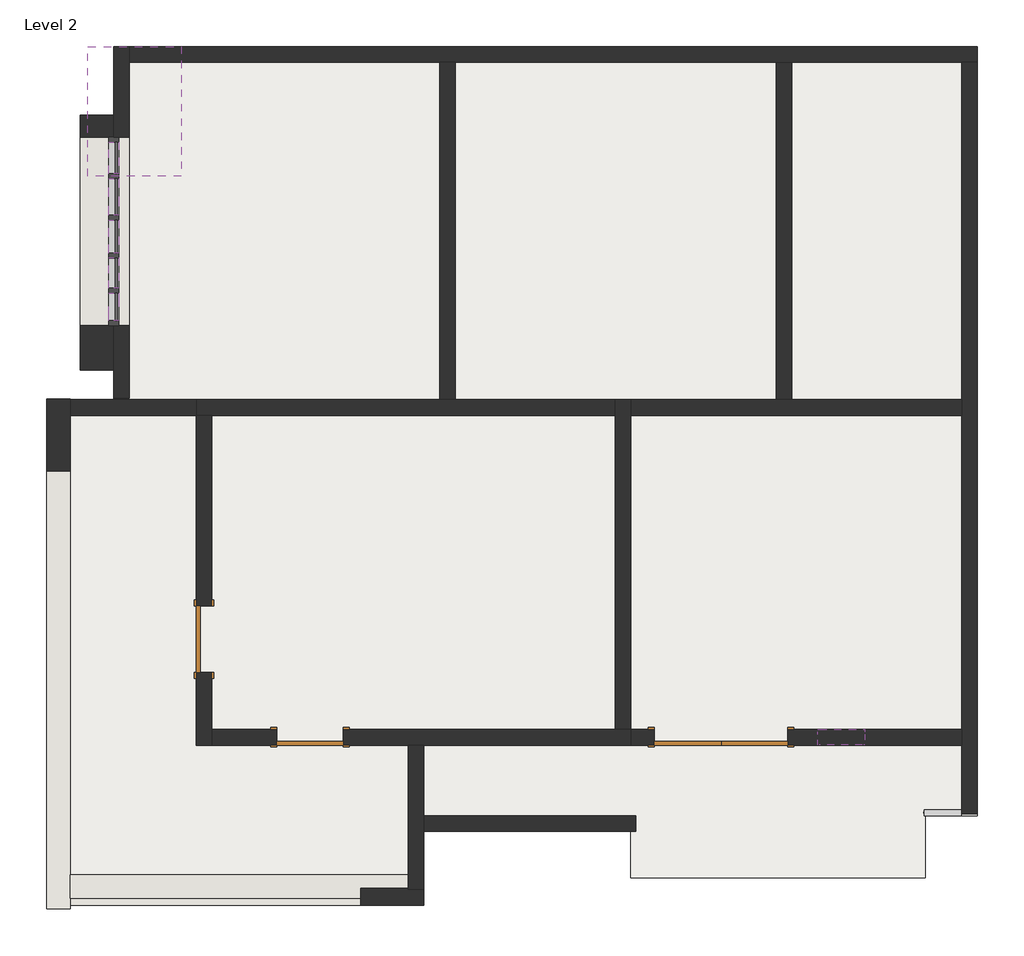
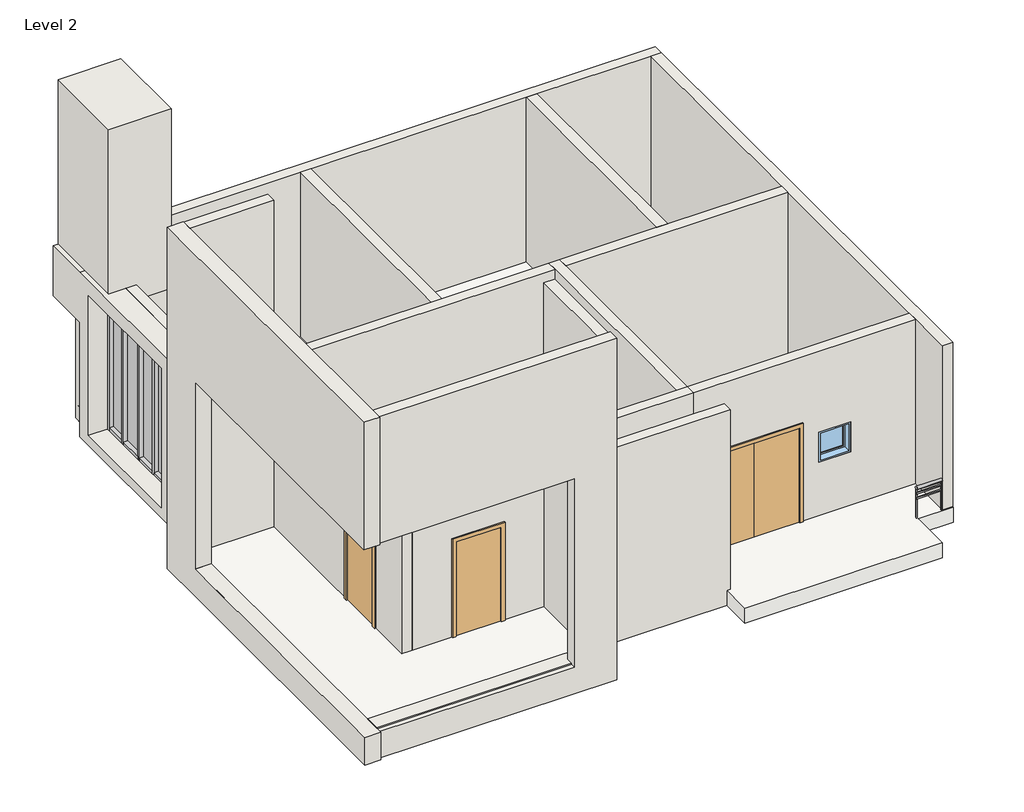
# One storey, incomplete: 19 walls, 16 members, 5 plates, 3 doors, 1 railing, 1 roof, 1 window.
"""IFC4 building model written with IfcOpenShell, lengths in millimetres."""

from ifc_helpers import new_model, si_unit, point, frame, origin, place, context, project, spatial, polyline, ellipse_curve, trimmed, outline, extrude, faceted_brep, transform, mapped, element, save
from ifc_brep_helpers import plane_surface, extruded_surface, advanced_brep
from components import door_aae36eb6, door_ef9e9df2, member_dc106669, member_39486dda, member_2b79973d, member_de12f0f3, member_76ec7c80, member_ae973821, member_2680e53c, system_panel_glazed_213fa7e9, system_panel_glazed_fd82e51e, system_panel_glazed_76cbe525, system_panel_glazed_7e745cad, system_panel_glazed_6096bcca, walls_1_walls_1_c089fa37, walls_2_walls_2_432dc62d, walls_3_walls_3_a2c954b4, walls_4_walls_4_aecb3609, walls_5_walls_5_067f5539, window_6846e476

model = new_model("IFC4")

# Units and contexts
model_context = context("Model", 3, world=origin())
ifc_project = project(units=[si_unit("LENGTHUNIT", "METRE", prefix="MILLI")], contexts=[model_context])

# Site, building, storey
site = spatial("IfcSite", under=ifc_project)
building = spatial("IfcBuilding", under=site)
storey = spatial("IfcBuildingStorey", under=building, Name="Level 2", Elevation=3657.6)

# Doors
placement = place(None, origin())
door_shape = door_aae36eb6(model_context)
element("IfcDoor", 1, ObjectType="Door-Double-Flush_Panel : 68\" x 80\"", at=placement, inside=storey, context=model_context, shape_type="MappedRepresentation", body=[
    mapped(door_shape, transform((-3927.8833771, 2417.2609482, 3860.8), x_axis=(-1.0, 0.0, 0.0), y_axis=(0.0, -1.0, 0.0), z_axis=(0.0, 0.0, 1.0))),
])
door_2_shape = door_ef9e9df2(model_context)
element("IfcDoor", 2, ObjectType="Single-Flush : 34\" x 80\"", at=placement, inside=storey, context=model_context, shape_type="MappedRepresentation", body=[
    mapped(door_2_shape, transform((-10617.8932708, 3687.2609482, 3860.8), x_axis=(0.0, 1.0, 0.0), y_axis=(-1.0, 0.0, 0.0), z_axis=(0.0, 0.0, 1.0))),
])
element("IfcDoor", 3, ObjectType="Single-Flush : 34\" x 80\"", at=placement, inside=storey, context=model_context, shape_type="MappedRepresentation", body=[
    mapped(door_2_shape, transform((-9246.2932708, 2417.2609482, 3860.8), x_axis=(-1.0, 0.0, 0.0), y_axis=(0.0, -1.0, 0.0), z_axis=(0.0, 0.0, 1.0))),
])

# Members
member_shape = member_dc106669(model_context)
element("IfcMember", 4, ObjectType="Rectangular Mullion : 2.5\" x 5\" rectangular", at=placement, inside=storey, context=model_context, shape_type="MappedRepresentation", body=[
    mapped(member_shape, transform((-11786.2932708, 10123.5597172, 4163.611227), x_axis=(0.0, 0.0, -1.0), y_axis=(-1.0, 0.0, 0.0), z_axis=(0.0, 1.0, 0.0))),
])
member_2_shape = member_39486dda(model_context)
element("IfcMember", 5, ObjectType="Rectangular Mullion : 2.5\" x 5\" rectangular", at=placement, inside=storey, context=model_context, shape_type="MappedRepresentation", body=[
    mapped(member_2_shape, transform((-11786.2932708, 9113.9097172, 4163.611227), x_axis=(0.0, 0.0, -1.0), y_axis=(-1.0, 0.0, 0.0), z_axis=(0.0, 1.0, 0.0))),
])
member_3_shape = member_2b79973d(model_context)
element("IfcMember", 6, ObjectType="Rectangular Mullion : 2.5\" x 5\" rectangular", at=placement, inside=storey, context=model_context, shape_type="MappedRepresentation", body=[
    mapped(member_3_shape, transform((-11786.2932708, 9647.3097172, 4163.611227), x_axis=(0.0, 0.0, -1.0), y_axis=(-1.0, 0.0, 0.0), z_axis=(0.0, 1.0, 0.0))),
])
member_4_shape = member_de12f0f3(model_context)
element("IfcMember", 7, ObjectType="Rectangular Mullion : 2.5\" x 5\" rectangular", at=placement, inside=storey, context=model_context, shape_type="MappedRepresentation", body=[
    mapped(member_4_shape, transform((-11786.2932708, 8622.8430505, 4163.611227), x_axis=(0.0, 0.0, -1.0), y_axis=(-1.0, 0.0, 0.0), z_axis=(0.0, 1.0, 0.0))),
])
member_5_shape = member_76ec7c80(model_context)
element("IfcMember", 8, ObjectType="Rectangular Mullion : 2.5\" x 5\" rectangular", at=placement, inside=storey, context=model_context, shape_type="MappedRepresentation", body=[
    mapped(member_5_shape, transform((-11786.2932708, 8169.8763839, 4163.611227), x_axis=(0.0, 0.0, -1.0), y_axis=(-1.0, 0.0, 0.0), z_axis=(0.0, 1.0, 0.0))),
])
member_6_shape = member_ae973821(model_context)
element("IfcMember", 9, ObjectType="Rectangular Mullion : 2.5\" x 5\" rectangular", at=placement, inside=storey, context=model_context, shape_type="MappedRepresentation", body=[
    mapped(member_6_shape, transform((-11786.2932708, 9679.0597172, 4163.611227), x_axis=(0.0, -1.0, 0.0), y_axis=(-1.0, 0.0, 0.0), z_axis=(0.0, 0.0, -1.0))),
])
element("IfcMember", 10, ObjectType="Rectangular Mullion : 2.5\" x 5\" rectangular", at=placement, inside=storey, context=model_context, shape_type="MappedRepresentation", body=[
    mapped(member_6_shape, transform((-11786.2932708, 8654.5930505, 4163.611227), x_axis=(0.0, -1.0, 0.0), y_axis=(-1.0, 0.0, 0.0), z_axis=(0.0, 0.0, -1.0))),
])
element("IfcMember", 11, ObjectType="Rectangular Mullion : 2.5\" x 5\" rectangular", at=placement, inside=storey, context=model_context, shape_type="MappedRepresentation", body=[
    mapped(member_6_shape, transform((-11786.2932708, 9145.6597172, 4163.611227), x_axis=(0.0, -1.0, 0.0), y_axis=(-1.0, 0.0, 0.0), z_axis=(0.0, 0.0, -1.0))),
])
element("IfcMember", 12, ObjectType="Rectangular Mullion : 2.5\" x 5\" rectangular", at=placement, inside=storey, context=model_context, shape_type="MappedRepresentation", body=[
    mapped(member_6_shape, transform((-11786.2932708, 8201.6263839, 4163.611227), x_axis=(0.0, -1.0, 0.0), y_axis=(-1.0, 0.0, 0.0), z_axis=(0.0, 0.0, -1.0))),
])
element("IfcMember", 13, ObjectType="Rectangular Mullion : 2.5\" x 5\" rectangular", at=placement, inside=storey, context=model_context, shape_type="MappedRepresentation", body=[
    mapped(member_4_shape, transform((-11786.2932708, 8233.3763839, 7010.4), x_axis=(0.0, 0.0, 1.0), y_axis=(-1.0, 0.0, 0.0), z_axis=(0.0, -1.0, 0.0))),
])
element("IfcMember", 14, ObjectType="Rectangular Mullion : 2.5\" x 5\" rectangular", at=placement, inside=storey, context=model_context, shape_type="MappedRepresentation", body=[
    mapped(member_2_shape, transform((-11786.2932708, 8686.3430505, 7010.4), x_axis=(0.0, 0.0, 1.0), y_axis=(-1.0, 0.0, 0.0), z_axis=(0.0, -1.0, 0.0))),
])
element("IfcMember", 15, ObjectType="Rectangular Mullion : 2.5\" x 5\" rectangular", at=placement, inside=storey, context=model_context, shape_type="MappedRepresentation", body=[
    mapped(member_3_shape, transform((-11786.2932708, 9177.4097172, 7010.4), x_axis=(0.0, 0.0, 1.0), y_axis=(-1.0, 0.0, 0.0), z_axis=(0.0, -1.0, 0.0))),
])
element("IfcMember", 16, ObjectType="Rectangular Mullion : 2.5\" x 5\" rectangular", at=placement, inside=storey, context=model_context, shape_type="MappedRepresentation", body=[
    mapped(member_shape, transform((-11786.2932708, 9710.8097172, 7010.4), x_axis=(0.0, 0.0, 1.0), y_axis=(-1.0, 0.0, 0.0), z_axis=(0.0, -1.0, 0.0))),
])
element("IfcMember", 17, ObjectType="Rectangular Mullion : 2.5\" x 5\" rectangular", at=placement, inside=storey, context=model_context, shape_type="MappedRepresentation", body=[
    mapped(member_5_shape, transform((-11786.2932708, 7812.1597172, 7010.4), x_axis=(0.0, 0.0, 1.0), y_axis=(-1.0, 0.0, 0.0), z_axis=(0.0, -1.0, 0.0))),
])
member_7_shape = member_2680e53c(model_context)
element("IfcMember", 18, ObjectType="Rectangular Mullion : 2.5\" x 5\" rectangular", at=placement, inside=storey, context=model_context, shape_type="MappedRepresentation", body=[
    mapped(member_7_shape, transform((-11786.2932708, 10187.0597172, 7010.4), x_axis=(0.0, 1.0, 0.0), y_axis=(-1.0, 0.0, 0.0), z_axis=(0.0, 0.0, 1.0))),
])
element("IfcMember", 19, ObjectType="Rectangular Mullion : 2.5\" x 5\" rectangular", at=placement, inside=storey, context=model_context, shape_type="MappedRepresentation", body=[
    mapped(member_7_shape, transform((-11786.2932708, 7748.6597172, 4163.611227), x_axis=(0.0, -1.0, 0.0), y_axis=(-1.0, 0.0, 0.0), z_axis=(0.0, 0.0, -1.0))),
])

# Plates
system_panel_glazed_shape = system_panel_glazed_213fa7e9(model_context)
element("IfcPlate", 20, ObjectType="System Panel : Glazed", at=placement, inside=storey, context=model_context, shape_type="MappedRepresentation", body=[
    mapped(system_panel_glazed_shape, transform((-11786.2932708, 9917.1847172, 4227.111227), x_axis=(0.0, -1.0, 0.0), y_axis=(1.0, 0.0, 0.0), z_axis=(0.0, 0.0, 1.0))),
])
system_panel_glazed_2_shape = system_panel_glazed_fd82e51e(model_context)
element("IfcPlate", 21, ObjectType="System Panel : Glazed", at=placement, inside=storey, context=model_context, shape_type="MappedRepresentation", body=[
    mapped(system_panel_glazed_2_shape, transform((-11786.2932708, 9412.3597172, 4227.111227), x_axis=(0.0, -1.0, 0.0), y_axis=(1.0, 0.0, 0.0), z_axis=(0.0, 0.0, 1.0))),
])
system_panel_glazed_3_shape = system_panel_glazed_76cbe525(model_context)
element("IfcPlate", 22, ObjectType="System Panel : Glazed", at=placement, inside=storey, context=model_context, shape_type="MappedRepresentation", body=[
    mapped(system_panel_glazed_3_shape, transform((-11786.2932708, 8900.1263839, 4227.111227), x_axis=(0.0, -1.0, 0.0), y_axis=(1.0, 0.0, 0.0), z_axis=(0.0, 0.0, 1.0))),
])
system_panel_glazed_4_shape = system_panel_glazed_7e745cad(model_context)
element("IfcPlate", 23, ObjectType="System Panel : Glazed", at=placement, inside=storey, context=model_context, shape_type="MappedRepresentation", body=[
    mapped(system_panel_glazed_4_shape, transform((-11786.2932708, 8428.1097172, 4227.111227), x_axis=(0.0, -1.0, 0.0), y_axis=(1.0, 0.0, 0.0), z_axis=(0.0, 0.0, 1.0))),
])
system_panel_glazed_5_shape = system_panel_glazed_6096bcca(model_context)
element("IfcPlate", 24, ObjectType="System Panel : Glazed", at=placement, inside=storey, context=model_context, shape_type="MappedRepresentation", body=[
    mapped(system_panel_glazed_5_shape, transform((-11786.2932708, 7991.0180505, 4227.111227), x_axis=(0.0, -1.0, 0.0), y_axis=(1.0, 0.0, 0.0), z_axis=(0.0, 0.0, 1.0))),
])

# Railing
element("IfcRailing", 25, ObjectType="Glass Panel - Bottom Fill", at=placement, inside=storey, context=model_context, shape_type="SolidModel", body=[
    advanced_brep(
    [(-818.4208756, 1401.4180656, 4572.0), (-818.4208756, 1477.6180656, 4572.0), (-1301.0208756, 1401.4180656, 4572.0), (-1301.0208756, 1477.6180656, 4572.0)],
    [
        (0, 1, ellipse_curve(frame((-818.4208756, 1439.5180656, 4572.0), z_axis=(1.0, 0.0, 0.0), x_axis=(0.0, 1.0, 0.0)), 38.1, 28.575)),
        (1, 0, ellipse_curve(frame((-818.4208756, 1439.5180656, 4572.0), z_axis=(1.0, 0.0, 0.0), x_axis=(0.0, 1.0, 0.0)), 38.1, 28.575)),
        (2, 3, ellipse_curve(frame((-1301.0208756, 1439.5180656, 4572.0), z_axis=(-1.0, 0.0, 0.0), x_axis=(0.0, 1.0, 0.0)), 38.1, 28.575)),
        (3, 2, ellipse_curve(frame((-1301.0208756, 1439.5180656, 4572.0), z_axis=(-1.0, 0.0, 0.0), x_axis=(0.0, 1.0, 0.0)), 38.1, 28.575)),
        (0, 2),
        (3, 1),
    ],
    [
        plane_surface(frame((-818.4208756, 1439.5180656, 4572.0), z_axis=(1.0, 0.0, 0.0), x_axis=(0.0, -1.0, 0.0))),
        plane_surface(frame((-1301.0208756, 1439.5180656, 4572.0), z_axis=(-1.0, 0.0, 0.0), x_axis=(0.0, -1.0, 0.0))),
        extruded_surface(trimmed(ellipse_curve(frame((-1301.0208756, 1439.5180656, 4572.0), z_axis=(1.0, 0.0, 0.0), x_axis=(0.0, 1.0, 0.0)), 38.1, 28.575), [point((-1301.0208756, 1401.4180656, 4572.0))], [point((-1301.0208756, 1477.6180656, 4572.0))], True, "CARTESIAN"), (482.5999999999999, 0.0, 0.0), 482.5999999999999),
        extruded_surface(trimmed(ellipse_curve(frame((-1301.0208756, 1439.5180656, 4572.0), z_axis=(1.0, 0.0, 0.0), x_axis=(0.0, 1.0, 0.0)), 38.1, 28.575), [point((-1301.0208756, 1477.6180656, 4572.0))], [point((-1301.0208756, 1401.4180656, 4572.0))], True, "CARTESIAN"), (482.5999999999999, 0.0, 0.0), 482.5999999999999),
    ],
    [
        (0, [[1, 2]]),
        (1, [[3, 4]]),
        (2, [[-1, 5, -4, 6]]),
        (3, [[-2, -6, -3, -5]]),
    ],
),
    extrude(outline(polyline([(-818.4208756, 1452.2180656), (-818.4208756, 1426.8180656), (-1301.0208756, 1426.8180656), (-1301.0208756, 1452.2180656), (-818.4208756, 1452.2180656)])), frame((0.0, 0.0, 4457.7), z_axis=(0.0, 0.0, 1.0), x_axis=(1.0, 0.0, 0.0)), (0.0, 0.0, 1.0), 25.4),
    extrude(outline(polyline([(-818.4208756, 1452.2180656), (-818.4208756, 1426.8180656), (-1301.0208756, 1426.8180656), (-1301.0208756, 1452.2180656), (-818.4208756, 1452.2180656)])), frame((0.0, 0.0, 4356.1), z_axis=(0.0, 0.0, 1.0), x_axis=(1.0, 0.0, 0.0)), (0.0, 0.0, 1.0), 25.4),
    extrude(outline(polyline([(-1288.3208756, 1449.0430656), (-1288.3208756, 1429.9930656), (-1307.3708756, 1429.9930656), (-1307.3708756, 1449.0430656), (-1288.3208756, 1449.0430656)])), frame((0.0, 0.0, 3657.6), z_axis=(0.0, 0.0, 1.0), x_axis=(1.0, 0.0, 0.0)), (0.0, 0.0, 1.0), 885.6788223),
    extrude(outline(polyline([(-812.0708756, 1449.0430656), (-812.0708756, 1429.9930656), (-831.1208756, 1429.9930656), (-831.1208756, 1449.0430656), (-812.0708756, 1449.0430656)])), frame((0.0, 0.0, 3657.6), z_axis=(0.0, 0.0, 1.0), x_axis=(1.0, 0.0, 0.0)), (0.0, 0.0, 1.0), 885.6788223),
])

# Roof
element("IfcRoof", 26, ObjectType="Generic - 12\"", at=placement, inside=storey, context=model_context, shape_type="SweptSolid", body=[
    extrude(outline(polyline([(-11786.2932708, 11358.0609482), (-610.2932708, 11358.0609482), (-610.2932708, 1401.2609482), (-1286.2833771, 1401.2609482), (-1286.2833771, 600.2635335), (-5096.2833771, 600.2635335), (-5096.2833771, 1401.2609482), (-7773.0932708, 1401.2609482), (-7773.0932708, 639.2609482), (-12345.0932708, 639.2609482), (-12345.0932708, 6786.0609482), (-11786.2932708, 6786.0609482), (-11786.2932708, 11358.0609482)])), frame((0.0, 0.0, 3657.6), z_axis=(0.0, 0.0, 1.0), x_axis=(1.0, 0.0, 0.0)), (0.0, 0.0, 1.0), 304.8),
])

# Walls
element("IfcWall", 27, ObjectType="Generic - 8\"", at=placement, inside=storey, context=model_context, shape_type="SweptSolid", body=[
    extrude(outline(polyline([(-5032.7833771, 1198.0609482), (-7773.0932708, 1198.0609482), (-7773.0932708, 1401.2609482), (-5032.7833771, 1401.2609482), (-5032.7833771, 1198.0609482)])), frame((0.0, 0.0, 3657.6), z_axis=(0.0, 0.0, 1.0), x_axis=(1.0, 0.0, 0.0)), (0.0, 0.0, 1.0), 3962.4),
])
element("IfcWall", 28, ObjectType="Generic - 8\"", at=placement, inside=storey, context=model_context, shape_type="Brep", body=[
    faceted_brep([(-10719.4932708, 6582.8609482, 3657.6), (-10719.4932708, 2315.6609482, 3657.6), (-10719.4932708, 2315.6609482, 7315.2), (-10719.4932708, 6582.8609482, 7315.2), (-10719.4932708, 3255.4609482, 3860.8), (-10719.4932708, 4119.0609482, 3860.8), (-10719.4932708, 4119.0609482, 5892.8), (-10719.4932708, 3255.4609482, 5892.8), (-10516.2932708, 6582.8609482, 3657.6), (-10516.2932708, 6582.8609482, 7315.2), (-10516.2932708, 2518.8609482, 7315.2), (-10516.2932708, 2315.6609482, 7315.2), (-10516.2932708, 2315.6609482, 3657.6), (-10516.2932708, 2518.8609482, 3657.6), (-10516.2932708, 3255.4609482, 3860.8), (-10516.2932708, 3255.4609482, 5892.8), (-10516.2932708, 4119.0609482, 5892.8), (-10516.2932708, 4119.0609482, 3860.8)], [[[0, 1, 2, 3], [4, 5, 6, 7]], [[8, 9, 10, 11, 12, 13], [14, 15, 16, 17]], [[1, 0, 8, 13, 12]], [[2, 1, 12, 11]], [[0, 3, 9, 8]], [[3, 2, 11, 10, 9]], [[5, 4, 14, 17]], [[6, 5, 17, 16]], [[7, 6, 16, 15]], [[4, 7, 15, 14]]]),
])
element("IfcWall", 29, ObjectType="Generic - 8\"", at=placement, inside=storey, context=model_context, shape_type="Brep", body=[
    faceted_brep([(-10516.2932708, 2315.6609482, 3657.6), (-7976.2932708, 2315.6609482, 3657.6), (-7773.0932708, 2315.6609482, 3657.6), (-5096.2833771, 2315.6609482, 3657.6), (-5096.2833771, 2315.6609482, 7315.2), (-10516.2932708, 2315.6609482, 7315.2), (-8814.4932708, 2315.6609482, 3860.8), (-9678.0932708, 2315.6609482, 3860.8), (-9678.0932708, 2315.6609482, 5892.8), (-8814.4932708, 2315.6609482, 5892.8), (-10516.2932708, 2518.8609482, 3657.6), (-10516.2932708, 2518.8609482, 7315.2), (-5299.4833771, 2518.8609482, 7315.2), (-5096.2833771, 2518.8609482, 7315.2), (-5096.2833771, 2518.8609482, 3657.6), (-5299.4833771, 2518.8609482, 3657.6), (-8814.4932708, 2518.8609482, 3860.8), (-8814.4932708, 2518.8609482, 5892.8), (-9678.0932708, 2518.8609482, 5892.8), (-9678.0932708, 2518.8609482, 3860.8)], [[[0, 1, 2, 3, 4, 5], [6, 7, 8, 9]], [[10, 11, 12, 13, 14, 15], [16, 17, 18, 19]], [[3, 2, 1, 0, 10, 15, 14]], [[0, 5, 11, 10]], [[4, 3, 14, 13]], [[5, 4, 13, 12, 11]], [[7, 6, 16, 19]], [[8, 7, 19, 18]], [[9, 8, 18, 17]], [[6, 9, 17, 16]]]),
])
element("IfcWall", 30, ObjectType="Generic - 8\"", at=placement, inside=storey, context=model_context, shape_type="Brep", body=[
    faceted_brep([(-5096.2833771, 2518.8609482, 3657.6), (-5096.2833771, 6582.8609482, 3657.6), (-5096.2833771, 6786.0609482, 3657.6), (-5096.2833771, 6786.0609482, 7315.2), (-5096.2833771, 6582.8609482, 7315.2), (-5096.2833771, 2518.8609482, 7315.2), (-5299.4833771, 2518.8609482, 3657.6), (-5299.4833771, 2518.8609482, 7315.2), (-5299.4833771, 6582.8609482, 7315.2), (-5299.4833771, 6786.0609482, 7315.2), (-5299.4833771, 6786.0609482, 3657.6), (-5299.4833771, 6582.8609482, 3657.6)], [[[0, 1, 2, 3, 4, 5]], [[6, 7, 8, 9, 10, 11]], [[2, 1, 0, 6, 11, 10]], [[0, 5, 7, 6]], [[3, 2, 10, 9]], [[5, 4, 3, 9, 8, 7]]]),
])
element("IfcWall", 31, ObjectType="Generic - 8\"", at=placement, inside=storey, context=model_context, shape_type="Brep", body=[
    faceted_brep([(-5299.4833771, 6786.0609482, 3657.6), (-7366.6932708, 6786.0609482, 3657.6), (-7569.8932708, 6786.0609482, 3657.6), (-10719.4932708, 6786.0609482, 3657.6), (-10719.4932708, 6786.0609482, 7315.2), (-7569.8932708, 6786.0609482, 7315.2), (-7366.6932708, 6786.0609482, 7315.2), (-5299.4833771, 6786.0609482, 7315.2), (-5299.4833771, 6582.8609482, 3657.6), (-5299.4833771, 6582.8609482, 7315.2), (-10516.2932708, 6582.8609482, 7315.2), (-10719.4932708, 6582.8609482, 7315.2), (-10719.4932708, 6582.8609482, 3657.6), (-10516.2932708, 6582.8609482, 3657.6)], [[[0, 1, 2, 3, 4, 5, 6, 7]], [[8, 9, 10, 11, 12, 13]], [[3, 2, 1, 0, 8, 13, 12]], [[0, 7, 9, 8]], [[4, 3, 12, 11]], [[7, 6, 5, 4, 11, 10, 9]]]),
])
element("IfcWall", 32, ObjectType="Generic - 8\"", at=placement, inside=storey, context=model_context, shape_type="Brep", body=[
    faceted_brep([(-10719.4932708, 6786.0609482, 3657.6), (-12345.0932708, 6786.0609482, 3657.6), (-12345.0932708, 6786.0609482, 10617.2441528), (-10719.4932708, 6786.0609482, 10617.2441528), (-10719.4932708, 6786.0609482, 7315.2), (-10719.4932708, 6582.8609482, 3657.6), (-10719.4932708, 6582.8609482, 7315.2), (-10719.4932708, 6582.8609482, 10617.2441528), (-12345.0932708, 6582.8609482, 10617.2441528), (-12345.0932708, 6582.8609482, 9753.6), (-12345.0932708, 6582.8609482, 7315.2), (-12345.0932708, 6582.8609482, 3657.6)], [[[0, 1, 2, 3, 4]], [[5, 6, 7, 8, 9, 10, 11]], [[1, 0, 5, 11]], [[3, 2, 8, 7]], [[2, 1, 11, 10, 9, 8]], [[0, 4, 3, 7, 6, 5]]]),
])
element("IfcWall", 33, ObjectType="Generic - 8\"", at=placement, inside=storey, context=model_context, shape_type="Brep", body=[
    faceted_brep([(-7773.0932708, 449.3705335, 3657.6), (-7773.0932708, 1198.0609482, 3657.6), (-7773.0932708, 1401.2609482, 3657.6), (-7773.0932708, 2315.6609482, 3657.6), (-7773.0932708, 2315.6609482, 10562.7595932), (-7773.0932708, 449.3705335, 10562.7595932), (-7976.2932708, 449.3705335, 3657.6), (-7976.2932708, 449.3705335, 10562.7595932), (-7976.2932708, 2315.6609482, 10562.7595932), (-7976.2932708, 2315.6609482, 3657.6)], [[[0, 1, 2, 3, 4, 5]], [[6, 7, 8, 9]], [[3, 2, 1, 0, 6, 9]], [[5, 4, 8, 7]], [[0, 5, 7, 6]], [[4, 3, 9, 8]]]),
])
element("IfcWall", 34, ObjectType="Generic - 8\"", at=placement, inside=storey, context=model_context, shape_type="Brep", body=[
    faceted_brep([(-11786.2932708, 11358.0609482, 7315.2), (-11786.2932708, 11358.0609482, 3657.6), (-11786.2932708, 11154.8609482, 3657.6), (-11786.2932708, 6811.4609482, 3657.6), (-11786.2932708, 6811.4609482, 7315.2), (-11786.2932708, 7748.6597172, 7010.4), (-11786.2932708, 7748.6597172, 4163.611227), (-11786.2932708, 10187.0597172, 4163.611227), (-11786.2932708, 10187.0597172, 7010.4), (-11583.0932708, 11358.0609482, 3657.6), (-11583.0932708, 11358.0609482, 7315.2), (-11583.0932708, 11154.8609482, 7315.2), (-11583.0932708, 6811.4609482, 7315.2), (-11583.0932708, 6811.4609482, 3657.6), (-11583.0932708, 11154.8609482, 3657.6), (-11583.0932708, 7748.6597172, 7010.4), (-11583.0932708, 10187.0597172, 7010.4), (-11583.0932708, 10187.0597172, 4163.611227), (-11583.0932708, 7748.6597172, 4163.611227)], [[[0, 1, 2, 3, 4], [5, 6, 7, 8]], [[9, 10, 11, 12, 13, 14], [15, 16, 17, 18]], [[3, 2, 1, 9, 14, 13]], [[4, 3, 13, 12]], [[0, 4, 12, 11, 10]], [[6, 5, 15, 18]], [[7, 6, 18, 17]], [[8, 7, 17, 16]], [[5, 8, 16, 15]], [[0, 10, 9, 1]]]),
])
element("IfcWall", 35, ObjectType="Generic - 8\"", at=placement, inside=storey, context=model_context, shape_type="Brep", body=[
    faceted_brep([(-11583.0932708, 11154.8609482, 7315.2), (-11583.0932708, 11154.8609482, 3657.6), (-7569.8932708, 11154.8609482, 3657.6), (-7366.6932708, 11154.8609482, 3657.6), (-3216.6833771, 11154.8609482, 3657.6), (-3013.4833771, 11154.8609482, 3657.6), (-813.4932708, 11154.8609482, 3657.6), (-610.2932708, 11154.8609482, 3657.6), (-610.2932708, 11154.8609482, 7315.2), (-813.4932708, 11154.8609482, 7315.2), (-3013.4833771, 11154.8609482, 7315.2), (-3216.6833771, 11154.8609482, 7315.2), (-7366.6932708, 11154.8609482, 7315.2), (-7569.8932708, 11154.8609482, 7315.2), (-11583.0932708, 11358.0609482, 3657.6), (-11583.0932708, 11358.0609482, 7315.2), (-610.2932708, 11358.0609482, 7315.2), (-610.2932708, 11358.0609482, 3657.6), (-813.4932708, 11358.0609482, 3657.6)], [[[0, 1, 2, 3, 4, 5, 6, 7, 8, 9, 10, 11, 12, 13]], [[14, 15, 16, 17, 18]], [[7, 6, 5, 4, 3, 2, 1, 14, 18, 17]], [[0, 13, 12, 11, 10, 9, 8, 16, 15]], [[7, 17, 16, 8]], [[0, 15, 14, 1]]]),
])
element("IfcWall", 36, ObjectType="Generic - 8\"", at=placement, inside=storey, context=model_context, shape_type="Brep", body=[
    faceted_brep([(-813.4932708, 11154.8609482, 7315.2), (-813.4932708, 11154.8609482, 3657.6), (-813.4932708, 6786.0609482, 3657.6), (-813.4932708, 6582.8609482, 3657.6), (-813.4932708, 2518.8609482, 3657.6), (-813.4932708, 2315.6609482, 3657.6), (-813.4932708, 1426.6609482, 3657.6), (-813.4932708, 1426.6609482, 7315.2), (-813.4932708, 2315.6609482, 7315.2), (-813.4932708, 2518.8609482, 7315.2), (-813.4932708, 6582.8609482, 7315.2), (-813.4932708, 6786.0609482, 7315.2), (-610.2932708, 11154.8609482, 3657.6), (-610.2932708, 11154.8609482, 7315.2), (-610.2932708, 1426.6609482, 7315.2), (-610.2932708, 1426.6609482, 3657.6)], [[[0, 1, 2, 3, 4, 5, 6, 7, 8, 9, 10, 11]], [[12, 13, 14, 15]], [[6, 5, 4, 3, 2, 1, 12, 15]], [[7, 6, 15, 14]], [[0, 11, 10, 9, 8, 7, 14, 13]], [[0, 13, 12, 1]]]),
])
element("IfcWall", 37, ObjectType="Generic - 8\"", at=placement, inside=storey, context=model_context, shape_type="SweptSolid", body=[
    extrude(outline(polyline([(3657.6, -5096.2833771), (3657.6, -813.4932708), (7315.2, -813.4932708), (7315.2, -5096.2833771), (3657.6, -5096.2833771)]), holes=[polyline([(3860.8, -4791.4833771), (5892.8, -4791.4833771), (5892.8, -3064.2833771), (3860.8, -3064.2833771), (3860.8, -4791.4833771)]), polyline([(5659.5979093, -2065.888324), (5049.9979093, -2065.888324), (5049.9979093, -2675.488324), (5659.5979093, -2675.488324), (5659.5979093, -2065.888324)])]), frame((0.0, 2315.6609482, 0.0), z_axis=(0.0, 1.0, 0.0), x_axis=(0.0, 0.0, 1.0)), (0.0, 0.0, 1.0), 203.2),
])
element("IfcWall", 38, ObjectType="Generic - 8\"", at=placement, inside=storey, context=model_context, shape_type="Brep", body=[
    faceted_brep([(-5096.2833771, 6582.8609482, 3657.6), (-813.4932708, 6582.8609482, 3657.6), (-813.4932708, 6582.8609482, 7315.2), (-5096.2833771, 6582.8609482, 7315.2), (-5096.2833771, 6786.0609482, 3657.6), (-5096.2833771, 6786.0609482, 7315.2), (-3216.6833771, 6786.0609482, 7315.2), (-3013.4833771, 6786.0609482, 7315.2), (-813.4932708, 6786.0609482, 7315.2), (-813.4932708, 6786.0609482, 3657.6), (-3013.4833771, 6786.0609482, 3657.6), (-3216.6833771, 6786.0609482, 3657.6)], [[[0, 1, 2, 3]], [[4, 5, 6, 7, 8, 9, 10, 11]], [[1, 0, 4, 11, 10, 9]], [[3, 2, 8, 7, 6, 5]], [[0, 3, 5, 4]], [[2, 1, 9, 8]]]),
])
element("IfcWall", 39, ObjectType="Generic - 8\"", at=placement, inside=storey, context=model_context, shape_type="SweptSolid", body=[
    extrude(outline(polyline([(-7366.6932708, 11154.8609482), (-7366.6932708, 6786.0609482), (-7569.8932708, 6786.0609482), (-7569.8932708, 11154.8609482), (-7366.6932708, 11154.8609482)])), frame((0.0, 0.0, 3657.6), z_axis=(0.0, 0.0, 1.0), x_axis=(1.0, 0.0, 0.0)), (0.0, 0.0, 1.0), 3657.6),
])
element("IfcWall", 40, ObjectType="Generic - 8\"", at=placement, inside=storey, context=model_context, shape_type="SweptSolid", body=[
    extrude(outline(polyline([(-3013.4833771, 11154.8609482), (-3013.4833771, 6786.0609482), (-3216.6833771, 6786.0609482), (-3216.6833771, 11154.8609482), (-3013.4833771, 11154.8609482)])), frame((0.0, 0.0, 3657.6), z_axis=(0.0, 0.0, 1.0), x_axis=(1.0, 0.0, 0.0)), (0.0, 0.0, 1.0), 3657.6),
])
walls_1_walls_1_shape = walls_1_walls_1_c089fa37(model_context)
element("IfcWall", 41, ObjectType="Walls 1 : Walls 1", at=placement, inside=storey, context=model_context, shape_type="MappedRepresentation", body=[
    mapped(walls_1_walls_1_shape, transform((0.0, 0.0, 0.0), x_axis=(1.0, 0.0, 0.0), y_axis=(0.0, 1.0, 0.0), z_axis=(0.0, 0.0, 1.0))),
])
walls_2_walls_2_shape = walls_2_walls_2_432dc62d(model_context)
element("IfcWall", 42, ObjectType="Walls 2 : Walls 2", at=placement, inside=storey, context=model_context, shape_type="MappedRepresentation", body=[
    mapped(walls_2_walls_2_shape, transform((0.0, 0.0, 0.0), x_axis=(1.0, 0.0, 0.0), y_axis=(0.0, 1.0, 0.0), z_axis=(0.0, 0.0, 1.0))),
])
walls_3_walls_3_shape = walls_3_walls_3_a2c954b4(model_context)
element("IfcWall", 43, ObjectType="Walls 3 : Walls 3", at=placement, inside=storey, context=model_context, shape_type="MappedRepresentation", body=[
    mapped(walls_3_walls_3_shape, transform((0.0, -38.1, 0.0), x_axis=(1.0, 0.0, 0.0), y_axis=(0.0, 1.0, 0.0), z_axis=(0.0, 0.0, 1.0))),
])
walls_4_walls_4_shape = walls_4_walls_4_aecb3609(model_context)
element("IfcWall", 44, ObjectType="Walls 4 : Walls 4", at=placement, inside=storey, context=model_context, shape_type="MappedRepresentation", body=[
    mapped(walls_4_walls_4_shape, transform((0.0, 0.0, 0.0), x_axis=(1.0, 0.0, 0.0), y_axis=(0.0, 1.0, 0.0), z_axis=(0.0, 0.0, 1.0))),
])
walls_5_walls_5_shape = walls_5_walls_5_067f5539(model_context)
element("IfcWall", 45, ObjectType="Walls 5 : Walls 5", at=placement, inside=storey, context=model_context, shape_type="MappedRepresentation", body=[
    mapped(walls_5_walls_5_shape, transform((0.0, 0.0, 0.0), x_axis=(1.0, 0.0, 0.0), y_axis=(0.0, 1.0, 0.0), z_axis=(0.0, 0.0, 1.0))),
])

# Window
window_shape = window_6846e476(model_context)
element("IfcWindow", 46, ObjectType="Fixed : 24\" x 24\"", at=placement, inside=storey, context=model_context, shape_type="MappedRepresentation", body=[
    mapped(window_shape, transform((-2332.588324, 2417.2609482, 4135.5979093), x_axis=(1.0, 0.0, 0.0), y_axis=(0.0, 1.0, 0.0), z_axis=(0.0, 0.0, 1.0))),
])

save(model, "model.ifc")

# Revit data of these elements
# Type "Door-Double-Flush_Panel : 68\" x 80\""
#   Type Mark = "9"
#   Construction Type Id = "DOOR"
#   Assembly Code = "C1020"
#   Analytic Construction = "Wooden"
#   Thickness = 0' - 2"
#   Thermal Resistance (R) = 2.5876 (h·ft²·°F)/BTU
#   Swing Angle [instance default] = 90.00°
#   Panel Width = 2' - 10"
#   Heat Transfer Coefficient (U) = 0.3865 BTU/(h·ft²·°F)
#   Height = 6' - 8"
#   Trim Projection Ext = 0' - 1"
#   Trim Projection Int = 0' - 1"
#   Trim Width = 0' - 3"
#   Width = 5' - 8"
#   Define Thermal Properties by = 1
#   Panel Material = Wood - Birch - Solid Stained Light Low Gloss
#   Trim Material = Paint - Sienna
#   Visual Light Transmittance = 0
#   Solar Heat Gain Coefficient = 0
#   Function = (empty or 0)
#   Wall Closure = (empty or 0)
# Type "Single-Flush : 34\" x 80\""
#   Type Mark = "7"
#   Construction Type Id = "MDOOR"
#   Assembly Code = "C1020"
#   Analytic Construction = "Metal"
#   Thickness = 0' - 2"
#   Heat Transfer Coefficient (U) = 0.651978 BTU/(h·ft²·°F)
#   Height = 6' - 8"
#   Trim Projection Ext = 0' - 1"
#   Trim Projection Int = 0' - 1"
#   Trim Width = 0' - 3"
#   Width = 2' - 10"
#   Define Thermal Properties by = 1
#   Door Material = Door - Panel
#   Frame Material = Door - Frame
#   Visual Light Transmittance = 0
#   Solar Heat Gain Coefficient = 0
#   Function = (empty or 0)
#   Wall Closure = (empty or 0)
# Type "Rectangular Mullion : 2.5\" x 5\" rectangular"
#   built-in parameter 1007304 = 0.416667 (stored number, unit not read)
#   built-in parameter 1007301 = 0.104167 (stored number, unit not read)
#   built-in parameter 1007300 = 0.104167 (stored number, unit not read)
# Type "System Panel : Glazed"
#   Construction Type Id = "GSP4R"
#   Analytic Construction = "1/8 in Pilkington single glazing"
#   Visual Light Transmittance = 0.9
#   Solar Heat Gain Coefficient = 0.86
#   Heat Transfer Coefficient (U) = 1.18115 BTU/(h·ft²·°F)
# Type "Glass Panel - Bottom Fill"
#   Assembly Code = "C2010400"
#   built-in parameter 1008612 = 0.0416667 (stored number, unit not read)
#   built-in parameter 1008611 = 0.0416667 (stored number, unit not read)
#   built-in parameter 1008609 = 0.333333 (stored number, unit not read)
#   built-in parameter 1008604 = 0.166667 (stored number, unit not read)
#   built-in parameter 1008603 = 0.166667 (stored number, unit not read)
#   Railing Height = 3' - 0"
#   built-in parameter 1008630 = 2
#   built-in parameter 1008610 = 2
#   built-in parameter 1008618 = Baluster - Square : 3/4"
# Type "Generic - 12\""
#   Assembly Code = "B1020"
#   Layers, outside or top first: 1' - 0" no material (function 1)
# Type "Generic - 8\""
#   Assembly Code = "B2010"
#   Layers, outside or top first: 0' - 8" no material (function 1)
# Type "Fixed : 24\" x 24\""
#   Type Mark = "3"
#   Construction Type Id = "GSP4R"
#   Assembly Code = "B2020100"
#   Analytic Construction = "1/8 in Pilkington single glazing"
#   Visual Light Transmittance = 0.9
#   Solar Heat Gain Coefficient = 0.78
#   Heat Transfer Coefficient (U) = 0.6496 BTU/(h·ft²·°F)
#   Height = 2' - 0"
#   Default Sill Height = 3' - 0"
#   Width = 2' - 0"
#   Window Inset = 0' - 0 3/4"
#   Define Thermal Properties by = 1
#   Glass Pane Material = Glass
#   Sash Material = Sash
#   Wall Closure = (empty or 0)
# Element 1 (IfcDoor, "Door-Double-Flush_Panel : 68\" x 80\"")
#   Swing Angle = 90.00°
#   Phase Created = New Construction
#   Materials on its faces: "Paint - Sienna", "Wood - Birch - Solid Stained Light Low Gloss"
# Elements 2, 3 (IfcDoor, "Single-Flush : 34\" x 80\"")
#   Phase Created = New Construction
#   Materials on its faces: "Door - Frame", "Door - Panel"
# Elements 4, 5, 6, 7, 8, 9, 10, 11, 12, 13, 14, 15, 16, 17, 18, 19 (IfcMember, "Rectangular Mullion : 2.5\" x 5\" rectangular")
#   Phase Created = New Construction
#   Materials on its faces: "Aluminum"
# Elements 20, 21, 22, 23, 24 (IfcPlate, "System Panel : Glazed")
#   Phase Created = New Construction
#   Materials on its faces: "Glass"
# Element 25 (IfcRailing, "Glass Panel - Bottom Fill")
#   Phase Created = New Construction
# Element 26 (IfcRoof, "Generic - 12\"")
#   built-in parameter 1001705 = 13 (stored number, unit not read)
#   built-in parameter 1001710 = 33615
#   Phase Created = New Construction
#   Materials on its faces: "Default Roof"
# Element 27 (IfcWall, "Generic - 8\"")
#   Top Offset = 0' - 0"
#   Base Offset = 0' - 0"
#   Unconnected Height = 13' - 0"
#   wall height = 13' - 0"
#   Phase Created = New Construction
#   Base Constraint = Level 2
#   Materials on its faces: "Default Wall"
# Elements 28, 29, 30, 31, 34, 35, 36, 37, 38, 39, 40 (IfcWall, "Generic - 8\"")
#   Top Offset = 0' - 0"
#   Base Offset = 0' - 0"
#   Unconnected Height = 12' - 0"
#   wall height = 12' - 0"
#   Phase Created = New Construction
#   Base Constraint = Level 2
#   Materials on its faces: "Default Wall"
# Element 32 (IfcWall, "Generic - 8\"")
#   Top Offset = 0' - 0"
#   Base Offset = 0' - 0"
#   Unconnected Height = 22' - 10.00174"
#   wall height = 22' - 10.00174"
#   Phase Created = New Construction
#   Base Constraint = Level 2
#   Materials on its faces: "Default Wall"
# Element 33 (IfcWall, "Generic - 8\"")
#   Top Offset = 0' - 0"
#   Base Offset = 0' - 0"
#   Unconnected Height = 22' - 7.85668"
#   wall height = 22' - 7.85668"
#   Phase Created = New Construction
#   Base Constraint = Level 2
#   Materials on its faces: "Default Wall"
# Element 41 (IfcWall, "Walls 1 : Walls 1")
#   Phase Created = New Construction
#   Materials on its faces: "Default Wall"
# Element 42 (IfcWall, "Walls 2 : Walls 2")
#   Phase Created = New Construction
#   Materials on its faces: "Default Wall"
# Element 43 (IfcWall, "Walls 3 : Walls 3")
#   Phase Created = New Construction
#   Materials on its faces: "Default Wall"
# Element 44 (IfcWall, "Walls 4 : Walls 4")
#   Phase Created = New Construction
#   Materials on its faces: "Default Wall"
# Element 45 (IfcWall, "Walls 5 : Walls 5")
#   Phase Created = New Construction
#   Materials on its faces: "Default Wall"
# Element 46 (IfcWindow, "Fixed : 24\" x 24\"")
#   Mark = "3"
#   Phase Created = New Construction
#   Materials on its faces: "Sash", "Glass"
# Materials
#   "Wood - Birch - Solid Stained Light Low Gloss": class "Wood", colour RGB 210 159 95, transparency 0, Cost = 0
#   "Paint - Sienna": colour RGB 118 70 51, transparency 0, Cost = 0
#   "Door - Panel": class "Wood", colour RGB 210 159 95, transparency 0
#   "Door - Frame": colour RGB 118 70 51, transparency 0
#   "Glass": class "Glass", colour RGB 0 128 192, transparency 0.75, Description = "Soda Lime Glass", Cost = 0
#   "Sash": class "Wood", colour RGB 224 178 126, transparency 0
#   "Aluminum": class "Metal", colour RGB 247 247 247, transparency 0, Description = "Aluminum 6061", Cost = 0
#   "Default Roof": colour RGB 88 101 114, transparency 0
#   "Default Wall": colour RGB 128 128 128, transparency 0
